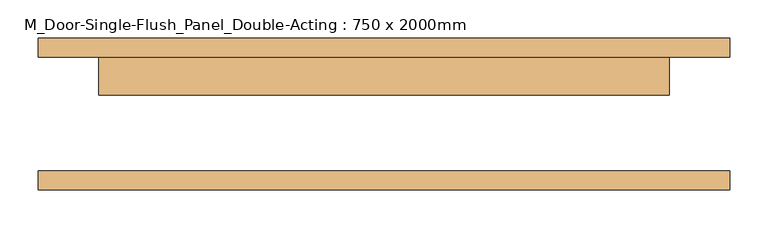
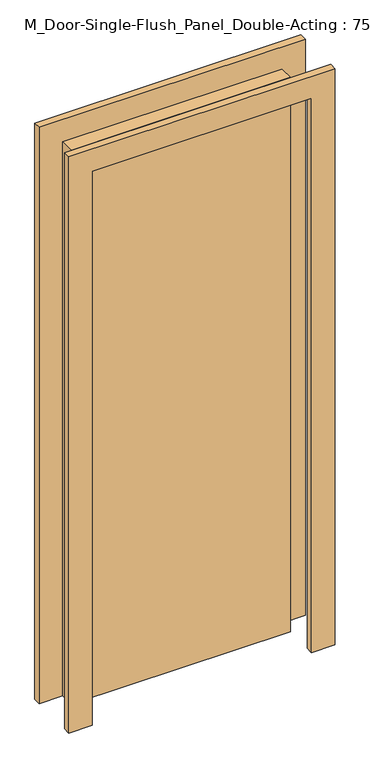
"""IFC4 building model written with IfcOpenShell, lengths in millimetres: door geometry, M_Door-Single-Flush_Panel_Double-Acting : 750 x 2000mm."""

from ifc_helpers import new_model, si_unit, frame, origin, origin_with_axes, place, context, project, spatial, polyline, outline, extrude, source, transform, mapped, element, save


def m_door_single_flush_panel_double_acting_750_x_2000mm_e3d998e5(model_context):
    return source(origin(), model_context, "Body", "SweptSolid", [
        extrude(outline(polyline([(375.0, 25.0), (-375.0, 25.0), (-375.0, 75.0), (375.0, 75.0), (375.0, 25.0)])), origin_with_axes(), (0.0, 0.0, 1.0), 2000.0),
        extrude(outline(polyline([(2080.0, 455.0), (2080.0, -455.0), (0.0, -455.0), (0.0, -375.0), (2000.0, -375.0), (2000.0, 375.0), (0.0, 375.0), (0.0, 455.0), (2080.0, 455.0)])), frame((0.0, -100.0, 0.0), z_axis=(0.0, 1.0, 0.0), x_axis=(0.0, 0.0, 1.0)), (0.0, 0.0, 1.0), 25.0),
        extrude(outline(polyline([(2080.0, -455.0), (0.0, -455.0), (0.0, -375.0), (2000.0, -375.0), (2000.0, 375.0), (0.0, 375.0), (0.0, 455.0), (2080.0, 455.0), (2080.0, -455.0)])), frame((0.0, 75.0, 0.0), z_axis=(0.0, 1.0, 0.0), x_axis=(0.0, 0.0, 1.0)), (0.0, 0.0, 1.0), 25.0),
    ])


if __name__ == "__main__":
    model = new_model("IFC4")
    model_context = context("Model", 3, world=origin())
    ifc_project = project(units=[si_unit("LENGTHUNIT", "METRE", prefix="MILLI")], contexts=[model_context])
    site = spatial("IfcSite", under=ifc_project)
    building = spatial("IfcBuilding", under=site)
    placement = place(None, origin())
    m_door_single_flush_panel_double_acting_750_x_2000mm_shape = m_door_single_flush_panel_double_acting_750_x_2000mm_e3d998e5(model_context)
    element("IfcDoor", 1, ObjectType="M_Door-Single-Flush_Panel_Double-Acting : 750 x 2000mm", at=placement, inside=building, context=model_context, shape_type="MappedRepresentation", body=[
        mapped(m_door_single_flush_panel_double_acting_750_x_2000mm_shape, transform((0.0, 0.0, 0.0), x_axis=(1.0, 0.0, 0.0), y_axis=(0.0, 1.0, 0.0), z_axis=(0.0, 0.0, 1.0))),
    ])
    save(model, "model.ifc")

# Revit data of these elements
# Type "M_Door-Single-Flush_Panel_Double-Acting : 750 x 2000mm"
#   Type Mark = "45"
#   Construction Type Id = "DOOR"
#   Assembly Code = "C1020300"
#   Analytic Construction = "Wooden"
#   Thickness = 50 mm
#   Thermal Resistance (R) = 0.455703 (m²·K)/W
#   Swing Angle [instance default] = 90.00°
#   Heat Transfer Coefficient (U) = 2.19465 W/(m²·K)
#   Height = 2000 mm
#   Trim Projection Ext. = 25 mm
#   Trim Projection Int. = 25 mm
#   Trim Width Ext. = 80 mm
#   Trim Width Int. = 80 mm
#   Width = 750 mm
#   Define Thermal Properties by = 1
#   Trim Material = Paint - Sienna
#   Panel Material = Wood - Birch - Solid Stained Light Low Gloss
#   Visual Light Transmittance = 0
#   Solar Heat Gain Coefficient = 0
#   Function = (empty or 0)
#   Wall Closure = (empty or 0)
# Element 1 (IfcDoor, "M_Door-Single-Flush_Panel_Double-Acting : 750 x 2000mm")
#   Materials on its faces: "Paint - Sienna", "Wood - Birch - Solid Stained Light Low Gloss"
# Materials
#   "Paint - Sienna": colour RGB 118 70 51, transparency 0, Cost = 0
#   "Wood - Birch - Solid Stained Light Low Gloss": class "Wood", colour RGB 210 159 95, transparency 0, Cost = 0
